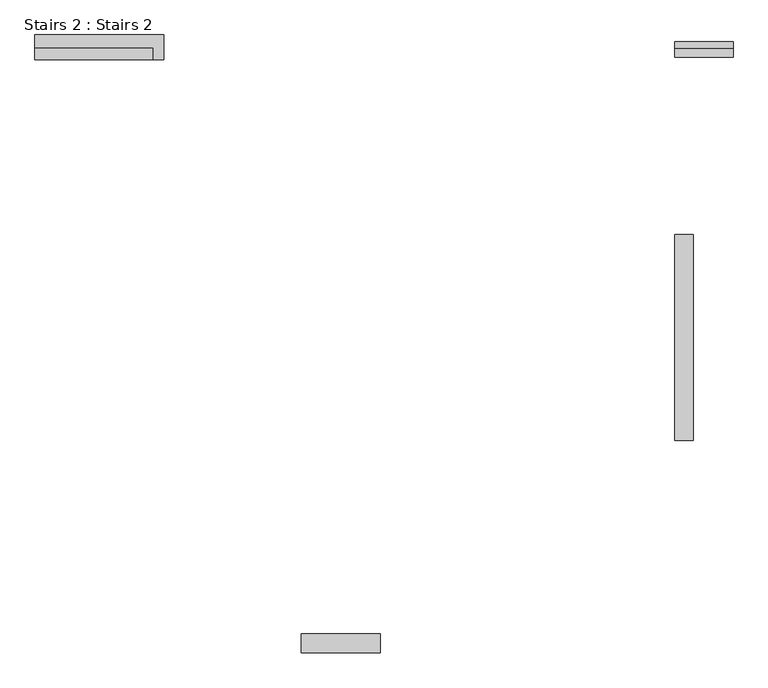
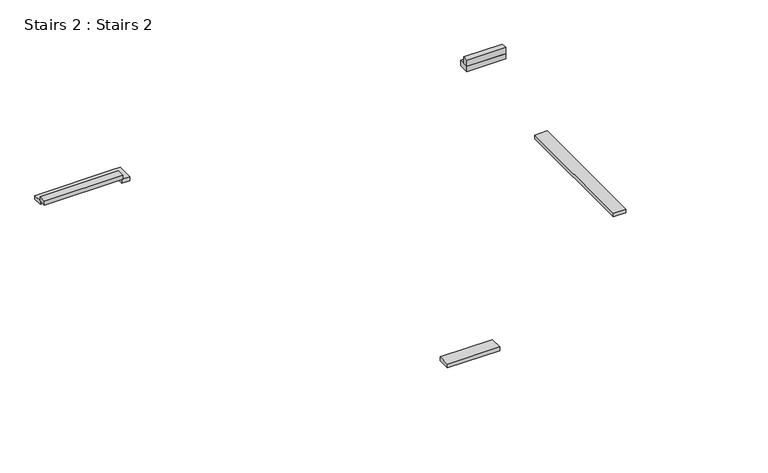
"""IFC4 building model written with IfcOpenShell, lengths in millimetres: stair geometry, Stairs 2 : Stairs 2."""

from ifc_helpers import new_model, si_unit, frame, origin, origin_with_axes, place, context, project, spatial, polyline, outline, extrude, source, transform, mapped, element, save


def stairs_2_stairs_2_b3d7acac(model_context):
    return source(origin(), model_context, "Body", "SweptSolid", [
        extrude(outline(polyline([(-44593.2041976, 12614.6483824), (-44593.2041976, 13078.7799463), (-42655.39796, 13078.7799463), (-42655.39796, 12614.6483824), (-44593.2041976, 12614.6483824)])), frame((0.0, 0.0, 449.9570313), z_axis=(0.0, 0.0, 1.0), x_axis=(1.0, 0.0, 0.0)), (0.0, 0.0, 1.0), 150.01875),
        extrude(outline(polyline([(-35422.74796, 27239.2621553), (-35422.74796, 27449.3394686), (-33990.9791975, 27449.3394686), (-33990.9791975, 27239.2621553), (-35422.74796, 27239.2621553)])), frame((0.0, 0.0, 200.025), z_axis=(0.0, 0.0, 1.0), x_axis=(1.0, 0.0, 0.0)), (0.0, 0.0, 1.0), 249.9320313),
        extrude(outline(polyline([(-35422.74796, 27239.2621553), (-35422.74796, 27628.0855094), (-33990.9791975, 27628.0855094), (-33990.9791975, 27239.2621553), (-35422.74796, 27239.2621553)])), origin_with_axes(), (0.0, 0.0, 1.0), 200.025),
        extrude(outline(polyline([(-34965.54796, 22884.744566), (-34965.54796, 17830.144566), (-35422.74796, 17830.144566), (-35422.74796, 22884.744566), (-34965.54796, 22884.744566)])), origin_with_axes(), (0.0, 0.0, 1.0), 150.01875),
        extrude(outline(polyline([(-48237.1755215, 27462.2116741), (-48237.1755215, 27176.4616741), (-51132.7755215, 27176.4616741), (-51132.7755215, 27462.2116741), (-48237.1755215, 27462.2116741)])), frame((0.0, 0.0, 300.0375), z_axis=(0.0, 0.0, 1.0), x_axis=(1.0, 0.0, 0.0)), (0.0, 0.0, 1.0), 149.9195313),
        extrude(outline(polyline([(-48262.5755215, 27792.4116741), (-47968.8111084, 27792.4116741), (-47968.8111084, 27185.8922457), (-48262.5755215, 27185.8922457), (-48262.5755215, 27462.2116741), (-51132.7755215, 27462.2116741), (-51132.7755215, 27792.4116741), (-48262.5755215, 27792.4116741)])), frame((0.0, 0.0, 150.01875), z_axis=(0.0, 0.0, 1.0), x_axis=(1.0, 0.0, 0.0)), (0.0, 0.0, 1.0), 150.01875),
    ])


if __name__ == "__main__":
    model = new_model("IFC4")
    model_context = context("Model", 3, world=origin())
    ifc_project = project(units=[si_unit("LENGTHUNIT", "METRE", prefix="MILLI")], contexts=[model_context])
    site = spatial("IfcSite", under=ifc_project)
    building = spatial("IfcBuilding", under=site)
    placement = place(None, origin())
    stairs_2_stairs_2_shape = stairs_2_stairs_2_b3d7acac(model_context)
    element("IfcStair", 1, ObjectType="Stairs 2 : Stairs 2", at=placement, inside=building, context=model_context, shape_type="MappedRepresentation", body=[
        mapped(stairs_2_stairs_2_shape, transform((0.0, 0.0, 0.0), x_axis=(1.0, 0.0, 0.0), y_axis=(0.0, 1.0, 0.0), z_axis=(0.0, 0.0, 1.0))),
    ])
    save(model, "model.ifc")
